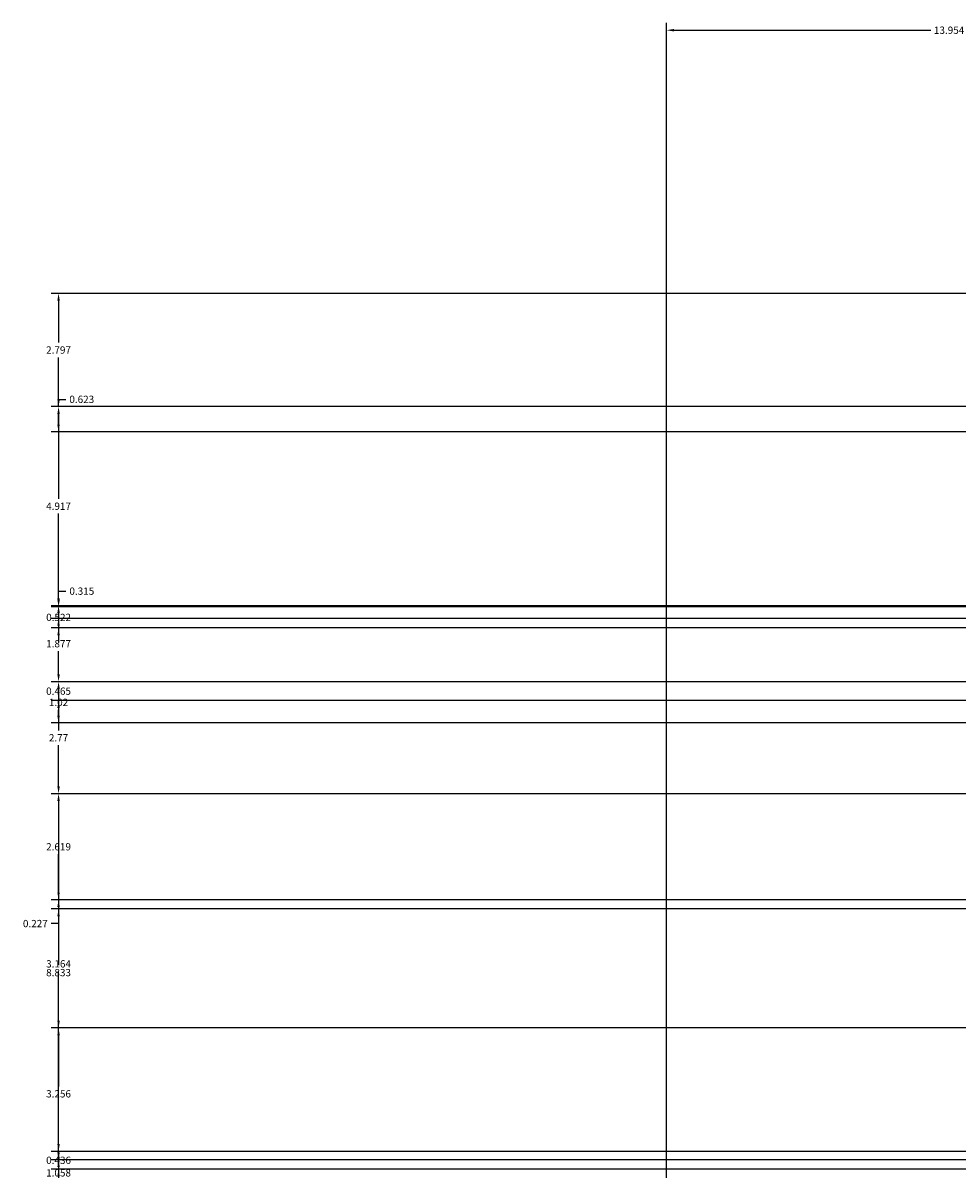
# Model space of a CAD drawing. Units: inches. Extents: x -10 to 130, y -32 to 34.
# Tile 5 of 22: x -10 to 13, y 6 to 34. Entities that reach past the tile are written whole.
import ezdxf

# ---------------------------------------------------------------- set-up
doc = ezdxf.new("R2010")
doc.units = ezdxf.units.IN
doc.header["$MEASUREMENT"] = 0
doc.layers.add('A-ANNO-DIMS', color=2, linetype='Continuous', lineweight=18)
doc.styles.get("Standard").update_dxf_attribs({"font": 'arial.ttf'})
doc.dimstyles.get("Standard").update_dxf_attribs({"dimtxt": 0.18, "dimasz": 0.18, "dimexe": 0.18, "dimexo": 0.0625, "dimgap": 0.09, "dimtad": 0, "dimtih": 1, "dimtoh": 1, "dimdec": 4, "dimzin": 0, "dimdsep": 46, "dimtxsty": 'Standard', "dimcen": 0.09, "dimadec": 0, "dimazin": 0, "dimtfac": 1, "dimtdec": 4, "dimtofl": 0, "dimtmove": 0, "dimatfit": 3, "dimfxl": 1, "dimtolj": 1, "dimtzin": 0, "dimarcsym": 0})

# ---------------------------------------------------------------- blocks, each defined once
blk = doc.blocks.new('*D11')
at = {"layer": 'A-ANNO-DIMS', "color": 0, "lineweight": -2, "transparency": 16777216}
for p, q in [((5.634, -12.739), (5.634, 33.879)), ((5.814, 33.699), (12.156, 33.699)), ((19.408, 33.699), (13.066, 33.699)), ((19.588, 19.547), (19.588, 33.879))]:
    blk.add_line(p, q, dxfattribs=at)
at = {"layer": 'A-ANNO-DIMS', "color": 0, "transparency": 16777216}
for points in [[(5.814, 33.729), (5.814, 33.669), (5.634, 33.699)], [(19.408, 33.729), (19.408, 33.669), (19.588, 33.699)]]:
    blk.add_solid(points, dxfattribs=at)
at = {"layer": 'Defpoints', "color": 0, "transparency": 16777216}
for p in [(19.588, 33.699), (19.588, 19.485), (5.634, -12.801)]:
    blk.add_point(p, dxfattribs=at)
at = {"layer": 'A-ANNO-DIMS', "color": 0, "transparency": 16777216, "insert": (12.611, 33.699), "char_height": 0.18, "attachment_point": 5}
blk.add_mtext('\\A1;13.954', dxfattribs=at)
blk = doc.blocks.new('*D34')
at = {"layer": 'A-ANNO-DIMS', "color": 0, "lineweight": -2, "transparency": 16777216}
for p, q in [((13.34, 6.007), (-9.564, 6.007)), ((-9.384, 5.827), (-9.384, 3.941)), ((-9.384, 1.691), (-9.384, 3.577)), ((70.835, 1.511), (-9.564, 1.511))]:
    blk.add_line(p, q, dxfattribs=at)
at = {"layer": 'A-ANNO-DIMS', "color": 0, "transparency": 16777216}
for points in [[(-9.414, 5.827), (-9.354, 5.827), (-9.384, 6.007)], [(-9.414, 1.691), (-9.354, 1.691), (-9.384, 1.511)]]:
    blk.add_solid(points, dxfattribs=at)
at = {"layer": 'Defpoints', "color": 0, "transparency": 16777216}
for p in [(-9.384, 6.007), (13.402, 6.007), (70.898, 1.511)]:
    blk.add_point(p, dxfattribs=at)
at = {"layer": 'A-ANNO-DIMS', "color": 0, "transparency": 16777216, "insert": (-9.384, 3.759), "char_height": 0.18, "attachment_point": 5}
blk.add_mtext('\\A1;4.497', dxfattribs=at)
blk = doc.blocks.new('*D35')
at = {"layer": 'A-ANNO-DIMS', "color": 0, "lineweight": -2, "transparency": 16777216}
for p, q in [((21.653, 14.841), (-9.564, 14.841)), ((-9.384, 14.661), (-9.384, 10.606)), ((-9.384, 6.187), (-9.384, 10.242)), ((13.34, 6.007), (-9.564, 6.007))]:
    blk.add_line(p, q, dxfattribs=at)
at = {"layer": 'A-ANNO-DIMS', "color": 0, "transparency": 16777216}
for points in [[(-9.414, 14.661), (-9.354, 14.661), (-9.384, 14.841)], [(-9.414, 6.187), (-9.354, 6.187), (-9.384, 6.007)]]:
    blk.add_solid(points, dxfattribs=at)
at = {"layer": 'Defpoints', "color": 0, "transparency": 16777216}
for p in [(-9.384, 14.841), (21.715, 14.841), (13.402, 6.007)]:
    blk.add_point(p, dxfattribs=at)
at = {"layer": 'A-ANNO-DIMS', "color": 0, "transparency": 16777216, "insert": (-9.384, 10.424), "char_height": 0.18, "attachment_point": 5}
blk.add_mtext('\\A1;8.833', dxfattribs=at)
blk = doc.blocks.new('*D36')
at = {"layer": 'A-ANNO-DIMS', "color": 0, "lineweight": -2, "transparency": 16777216}
for p, q in [((44.559, 17.607), (-9.564, 17.607)), ((-9.384, 17.427), (-9.384, 16.405)), ((-9.384, 15.021), (-9.384, 16.044)), ((21.653, 14.841), (-9.564, 14.841))]:
    blk.add_line(p, q, dxfattribs=at)
at = {"layer": 'A-ANNO-DIMS', "color": 0, "transparency": 16777216}
for points in [[(-9.414, 17.427), (-9.354, 17.427), (-9.384, 17.607)], [(-9.414, 15.021), (-9.354, 15.021), (-9.384, 14.841)]]:
    blk.add_solid(points, dxfattribs=at)
at = {"layer": 'Defpoints', "color": 0, "transparency": 16777216}
for p in [(-9.384, 17.607), (44.622, 17.607), (21.715, 14.841)]:
    blk.add_point(p, dxfattribs=at)
at = {"layer": 'A-ANNO-DIMS', "color": 0, "transparency": 16777216, "insert": (-9.384, 16.224), "char_height": 0.18, "attachment_point": 5}
blk.add_mtext('\\A1;2.77', dxfattribs=at)
blk = doc.blocks.new('*D37')
at = {"layer": 'A-ANNO-DIMS', "color": 0, "lineweight": -2, "transparency": 16777216}
for p, q in [((19.526, 19.485), (-9.564, 19.485)), ((-9.384, 19.305), (-9.384, 18.728)), ((-9.384, 17.787), (-9.384, 18.364)), ((44.559, 17.607), (-9.564, 17.607))]:
    blk.add_line(p, q, dxfattribs=at)
at = {"layer": 'A-ANNO-DIMS', "color": 0, "transparency": 16777216}
for points in [[(-9.414, 19.305), (-9.354, 19.305), (-9.384, 19.485)], [(-9.414, 17.787), (-9.354, 17.787), (-9.384, 17.607)]]:
    blk.add_solid(points, dxfattribs=at)
at = {"layer": 'Defpoints', "color": 0, "transparency": 16777216}
for p in [(-9.384, 19.485), (19.588, 19.485), (44.622, 17.607)]:
    blk.add_point(p, dxfattribs=at)
at = {"layer": 'A-ANNO-DIMS', "color": 0, "transparency": 16777216, "insert": (-9.384, 18.546), "char_height": 0.18, "attachment_point": 5}
blk.add_mtext('\\A1;1.877', dxfattribs=at)
blk = doc.blocks.new('*D38')
at = {"layer": 'A-ANNO-DIMS', "color": 0, "lineweight": -2, "transparency": 16777216}
for p, q in [((28.037, 24.402), (-9.564, 24.402)), ((-9.384, 24.222), (-9.384, 22.125)), ((-9.384, 19.665), (-9.384, 21.761)), ((19.526, 19.485), (-9.564, 19.485))]:
    blk.add_line(p, q, dxfattribs=at)
at = {"layer": 'A-ANNO-DIMS', "color": 0, "transparency": 16777216}
for points in [[(-9.414, 24.222), (-9.354, 24.222), (-9.384, 24.402)], [(-9.414, 19.665), (-9.354, 19.665), (-9.384, 19.485)]]:
    blk.add_solid(points, dxfattribs=at)
at = {"layer": 'Defpoints', "color": 0, "transparency": 16777216}
for p in [(-9.384, 24.402), (28.1, 24.402), (19.588, 19.485)]:
    blk.add_point(p, dxfattribs=at)
at = {"layer": 'A-ANNO-DIMS', "color": 0, "transparency": 16777216, "insert": (-9.384, 21.943), "char_height": 0.18, "attachment_point": 5}
blk.add_mtext('\\A1;4.917', dxfattribs=at)
blk = doc.blocks.new('*D39')
at = {"layer": 'A-ANNO-DIMS', "color": 0, "lineweight": -2, "transparency": 16777216}
for p, q in [((49.972, 27.199), (-9.564, 27.199)), ((-9.384, 27.019), (-9.384, 25.982)), ((-9.384, 24.582), (-9.384, 25.618)), ((28.037, 24.402), (-9.564, 24.402))]:
    blk.add_line(p, q, dxfattribs=at)
at = {"layer": 'A-ANNO-DIMS', "color": 0, "transparency": 16777216}
for points in [[(-9.414, 27.019), (-9.354, 27.019), (-9.384, 27.199)], [(-9.414, 24.582), (-9.354, 24.582), (-9.384, 24.402)]]:
    blk.add_solid(points, dxfattribs=at)
at = {"layer": 'Defpoints', "color": 0, "transparency": 16777216}
for p in [(-9.384, 27.199), (50.035, 27.199), (28.1, 24.402)]:
    blk.add_point(p, dxfattribs=at)
at = {"layer": 'A-ANNO-DIMS', "color": 0, "transparency": 16777216, "insert": (-9.384, 25.8), "char_height": 0.18, "attachment_point": 5}
blk.add_mtext('\\A1;2.797', dxfattribs=at)
blk = doc.blocks.new('*D74')
at = {"layer": 'A-ANNO-DIMS', "color": 0, "lineweight": -2, "transparency": 16777216}
for p, q in [((54.085, 17.607), (-9.564, 17.607)), ((-9.384, 17.427), (-9.384, 17.281)), ((-9.384, 16.771), (-9.384, 16.917)), ((55.856, 16.591), (-9.564, 16.591))]:
    blk.add_line(p, q, dxfattribs=at)
at = {"layer": 'A-ANNO-DIMS', "color": 0, "transparency": 16777216}
for points in [[(-9.414, 17.427), (-9.354, 17.427), (-9.384, 17.607)], [(-9.414, 16.771), (-9.354, 16.771), (-9.384, 16.591)]]:
    blk.add_solid(points, dxfattribs=at)
at = {"layer": 'Defpoints', "color": 0, "transparency": 16777216}
for p in [(54.147, 17.607), (-9.384, 16.591), (55.918, 16.591)]:
    blk.add_point(p, dxfattribs=at)
at = {"layer": 'A-ANNO-DIMS', "color": 0, "transparency": 16777216, "insert": (-9.384, 17.099), "char_height": 0.18, "attachment_point": 5}
blk.add_mtext('\\A1;1.02', dxfattribs=at)
blk = doc.blocks.new('*D87')
at = {"layer": 'A-ANNO-DIMS', "color": 0, "lineweight": -2, "transparency": 16777216}
for p, q in [((49.884, 14.841), (-9.564, 14.841)), ((-9.384, 14.661), (-9.384, 13.713)), ((-9.384, 12.402), (-9.384, 13.35)), ((49.884, 12.222), (-9.564, 12.222))]:
    blk.add_line(p, q, dxfattribs=at)
at = {"layer": 'A-ANNO-DIMS', "color": 0, "transparency": 16777216}
for points in [[(-9.414, 14.661), (-9.354, 14.661), (-9.384, 14.841)], [(-9.414, 12.402), (-9.354, 12.402), (-9.384, 12.222)]]:
    blk.add_solid(points, dxfattribs=at)
at = {"layer": 'Defpoints', "color": 0, "transparency": 16777216}
for p in [(49.946, 14.841), (-9.384, 12.222), (49.946, 12.222)]:
    blk.add_point(p, dxfattribs=at)
at = {"layer": 'A-ANNO-DIMS', "color": 0, "transparency": 16777216, "insert": (-9.384, 13.532), "char_height": 0.18, "attachment_point": 5}
blk.add_mtext('\\A1;2.619', dxfattribs=at)
blk = doc.blocks.new('*D88')
at = {"layer": 'A-ANNO-DIMS', "color": 0, "lineweight": -2, "transparency": 16777216}
for p, q in [((49.884, 12.222), (-9.564, 12.222)), ((-9.384, 12.042), (-9.384, 10.822)), ((-9.384, 9.238), (-9.384, 10.458)), ((49.884, 9.058), (-9.564, 9.058))]:
    blk.add_line(p, q, dxfattribs=at)
at = {"layer": 'A-ANNO-DIMS', "color": 0, "transparency": 16777216}
for points in [[(-9.414, 12.042), (-9.354, 12.042), (-9.384, 12.222)], [(-9.414, 9.238), (-9.354, 9.238), (-9.384, 9.058)]]:
    blk.add_solid(points, dxfattribs=at)
at = {"layer": 'Defpoints', "color": 0, "transparency": 16777216}
for p in [(49.946, 12.222), (-9.384, 9.058), (49.946, 9.058)]:
    blk.add_point(p, dxfattribs=at)
at = {"layer": 'A-ANNO-DIMS', "color": 0, "transparency": 16777216, "insert": (-9.384, 10.64), "char_height": 0.18, "attachment_point": 5}
blk.add_mtext('\\A1;3.164', dxfattribs=at)
blk = doc.blocks.new('*D89')
at = {"layer": 'A-ANNO-DIMS', "color": 0, "lineweight": -2, "transparency": 16777216}
for p, q in [((49.884, 9.058), (-9.564, 9.058)), ((-9.384, 8.878), (-9.384, 7.612)), ((-9.384, 5.982), (-9.384, 7.248)), ((49.884, 5.802), (-9.564, 5.802))]:
    blk.add_line(p, q, dxfattribs=at)
at = {"layer": 'A-ANNO-DIMS', "color": 0, "transparency": 16777216}
for points in [[(-9.414, 8.878), (-9.354, 8.878), (-9.384, 9.058)], [(-9.414, 5.982), (-9.354, 5.982), (-9.384, 5.802)]]:
    blk.add_solid(points, dxfattribs=at)
at = {"layer": 'Defpoints', "color": 0, "transparency": 16777216}
for p in [(49.946, 9.058), (-9.384, 5.802), (49.946, 5.802)]:
    blk.add_point(p, dxfattribs=at)
at = {"layer": 'A-ANNO-DIMS', "color": 0, "transparency": 16777216, "insert": (-9.384, 7.43), "char_height": 0.18, "attachment_point": 5}
blk.add_mtext('\\A1;3.256', dxfattribs=at)
blk = doc.blocks.new('*D90')
at = {"layer": 'A-ANNO-DIMS', "color": 0, "lineweight": -2, "transparency": 16777216}
for p, q in [((49.884, 5.802), (-9.564, 5.802)), ((-9.384, 5.622), (-9.384, 4.421)), ((-9.384, 2.855), (-9.384, 4.057)), ((49.884, 2.675), (-9.564, 2.675))]:
    blk.add_line(p, q, dxfattribs=at)
at = {"layer": 'A-ANNO-DIMS', "color": 0, "transparency": 16777216}
for points in [[(-9.414, 5.622), (-9.354, 5.622), (-9.384, 5.802)], [(-9.414, 2.855), (-9.354, 2.855), (-9.384, 2.675)]]:
    blk.add_solid(points, dxfattribs=at)
at = {"layer": 'Defpoints', "color": 0, "transparency": 16777216}
for p in [(49.946, 5.802), (-9.384, 2.675), (49.946, 2.675)]:
    blk.add_point(p, dxfattribs=at)
at = {"layer": 'A-ANNO-DIMS', "color": 0, "transparency": 16777216, "insert": (-9.384, 4.239), "char_height": 0.18, "attachment_point": 5}
blk.add_mtext('\\A1;3.127', dxfattribs=at)
blk = doc.blocks.new('*D95')
at = {"layer": 'A-ANNO-DIMS', "color": 0, "lineweight": -2, "transparency": 16777216}
for p, q in [((-9.384, 12.402), (-9.384, 12.582)), ((49.884, 12.222), (-9.564, 12.222)), ((49.884, 11.995), (-9.564, 11.995)), ((-9.384, 11.635), (-9.564, 11.635)), ((-9.384, 11.815), (-9.384, 11.635))]:
    blk.add_line(p, q, dxfattribs=at)
at = {"layer": 'A-ANNO-DIMS', "color": 0, "transparency": 16777216}
for points in [[(-9.414, 12.402), (-9.354, 12.402), (-9.384, 12.222)], [(-9.414, 11.815), (-9.354, 11.815), (-9.384, 11.995)]]:
    blk.add_solid(points, dxfattribs=at)
at = {"layer": 'Defpoints', "color": 0, "transparency": 16777216}
for p in [(49.946, 12.222), (-9.384, 11.995), (49.946, 11.995)]:
    blk.add_point(p, dxfattribs=at)
at = {"layer": 'A-ANNO-DIMS', "color": 0, "transparency": 16777216, "insert": (-9.957, 11.635), "char_height": 0.18, "attachment_point": 5}
blk.add_mtext('\\A1;0.227', dxfattribs=at)
blk = doc.blocks.new('*D98')
at = {"layer": 'A-ANNO-DIMS', "color": 0, "lineweight": -2, "transparency": 16777216}
for p, q in [((-9.384, 19.665), (-9.384, 19.845)), ((-9.384, 19.845), (-9.204, 19.845)), ((19.526, 19.485), (-9.564, 19.485)), ((19.785, 19.17), (-9.564, 19.17)), ((-9.384, 18.99), (-9.384, 18.81))]:
    blk.add_line(p, q, dxfattribs=at)
at = {"layer": 'A-ANNO-DIMS', "color": 0, "transparency": 16777216}
for points in [[(-9.414, 19.665), (-9.354, 19.665), (-9.384, 19.485)], [(-9.414, 18.99), (-9.354, 18.99), (-9.384, 19.17)]]:
    blk.add_solid(points, dxfattribs=at)
at = {"layer": 'Defpoints', "color": 0, "transparency": 16777216}
for p in [(-9.384, 19.485), (19.588, 19.485), (19.848, 19.17)]:
    blk.add_point(p, dxfattribs=at)
at = {"layer": 'A-ANNO-DIMS', "color": 0, "transparency": 16777216, "insert": (-8.809, 19.845), "char_height": 0.18, "attachment_point": 5}
blk.add_mtext('\\A1;0.315', dxfattribs=at)
blk = doc.blocks.new('*D101')
at = {"layer": 'A-ANNO-DIMS', "color": 0, "lineweight": -2, "transparency": 16777216}
for p, q in [((28.037, 24.402), (-9.564, 24.402)), ((-9.384, 24.402), (-9.384, 24.582)), ((-9.384, 24.582), (-9.204, 24.582)), ((-9.384, 23.959), (-9.384, 24.222)), ((28.602, 23.779), (-9.564, 23.779))]:
    blk.add_line(p, q, dxfattribs=at)
at = {"layer": 'A-ANNO-DIMS', "color": 0, "transparency": 16777216}
for points in [[(-9.414, 24.222), (-9.354, 24.222), (-9.384, 24.402)], [(-9.414, 23.959), (-9.354, 23.959), (-9.384, 23.779)]]:
    blk.add_solid(points, dxfattribs=at)
at = {"layer": 'Defpoints', "color": 0, "transparency": 16777216}
for p in [(-9.384, 24.402), (28.1, 24.402), (28.665, 23.779)]:
    blk.add_point(p, dxfattribs=at)
at = {"layer": 'A-ANNO-DIMS', "color": 0, "transparency": 16777216, "insert": (-8.81, 24.582), "char_height": 0.18, "attachment_point": 5}
blk.add_mtext('\\A1;0.623', dxfattribs=at)
blk = doc.blocks.new('*D104')
at = {"layer": 'A-ANNO-DIMS', "color": 0, "lineweight": -2, "transparency": 16777216}
for p, q in [((-9.383551, 19.637521), (-9.383551, 19.817521)), ((33.54566, 19.457521), (-9.563551, 19.457521)), ((33.931459, 18.935883), (-9.563551, 18.935883)), ((-9.383551, 18.755883), (-9.383551, 18.575883))]:
    blk.add_line(p, q, dxfattribs=at)
at = {"layer": 'A-ANNO-DIMS', "color": 0, "transparency": 16777216}
for points in [[(-9.413551, 19.637521), (-9.353551, 19.637521), (-9.383551, 19.457521)], [(-9.413551, 18.755883), (-9.353551, 18.755883), (-9.383551, 18.935883)]]:
    blk.add_solid(points, dxfattribs=at)
at = {"layer": 'Defpoints', "color": 0, "transparency": 16777216}
for p in [(-9.383551, 19.457521), (33.60816, 19.457521), (33.993959, 18.935883)]:
    blk.add_point(p, dxfattribs=at)
at = {"layer": 'A-ANNO-DIMS', "color": 0, "transparency": 16777216, "insert": (-9.383551, 19.196702), "char_height": 0.18, "attachment_point": 5}
blk.add_mtext('\\A1;0.522', dxfattribs=at)
blk = doc.blocks.new('*D110')
at = {"layer": 'A-ANNO-DIMS', "color": 0, "lineweight": -2, "transparency": 16777216}
for p, q in [((-9.383551, 17.787359), (-9.383551, 17.967359)), ((44.559228, 17.607359), (-9.563551, 17.607359)), ((45.040057, 17.142679), (-9.563551, 17.142679)), ((-9.383551, 16.962679), (-9.383551, 16.782679))]:
    blk.add_line(p, q, dxfattribs=at)
at = {"layer": 'A-ANNO-DIMS', "color": 0, "transparency": 16777216}
for points in [[(-9.413551, 17.787359), (-9.353551, 17.787359), (-9.383551, 17.607359)], [(-9.413551, 16.962679), (-9.353551, 16.962679), (-9.383551, 17.142679)]]:
    blk.add_solid(points, dxfattribs=at)
at = {"layer": 'Defpoints', "color": 0, "transparency": 16777216}
for p in [(-9.383551, 17.607359), (44.621728, 17.607359), (45.102557, 17.142679)]:
    blk.add_point(p, dxfattribs=at)
at = {"layer": 'A-ANNO-DIMS', "color": 0, "transparency": 16777216, "insert": (-9.383551, 17.375019), "char_height": 0.18, "attachment_point": 5}
blk.add_mtext('\\A1;0.465', dxfattribs=at)
blk = doc.blocks.new('*D113')
at = {"layer": 'A-ANNO-DIMS', "color": 0, "lineweight": -2, "transparency": 16777216}
for p, q in [((13.34, 6.007), (-9.564, 6.007)), ((-9.384, 5.827), (-9.384, 5.66)), ((-9.384, 5.13), (-9.384, 5.297)), ((14.67, 4.95), (-9.564, 4.95))]:
    blk.add_line(p, q, dxfattribs=at)
at = {"layer": 'A-ANNO-DIMS', "color": 0, "transparency": 16777216}
for points in [[(-9.414, 5.827), (-9.354, 5.827), (-9.384, 6.007)], [(-9.414, 5.13), (-9.354, 5.13), (-9.384, 4.95)]]:
    blk.add_solid(points, dxfattribs=at)
at = {"layer": 'Defpoints', "color": 0, "transparency": 16777216}
for p in [(-9.384, 6.007), (13.402, 6.007), (14.732, 4.95)]:
    blk.add_point(p, dxfattribs=at)
at = {"layer": 'A-ANNO-DIMS', "color": 0, "transparency": 16777216, "insert": (-9.384, 5.478), "char_height": 0.18, "attachment_point": 5}
blk.add_mtext('\\A1;1.058', dxfattribs=at)
blk = doc.blocks.new('*D115')
at = {"layer": 'A-ANNO-DIMS', "color": 0, "lineweight": -2, "transparency": 16777216}
for p, q in [((26.336, 6.007), (-9.564, 6.007)), ((-9.384, 5.827), (-9.384, 4.151)), ((-9.384, 2.111), (-9.384, 3.787)), ((26.336, 1.931), (-9.564, 1.931))]:
    blk.add_line(p, q, dxfattribs=at)
at = {"layer": 'A-ANNO-DIMS', "color": 0, "transparency": 16777216}
for points in [[(-9.414, 5.827), (-9.354, 5.827), (-9.384, 6.007)], [(-9.414, 2.111), (-9.354, 2.111), (-9.384, 1.931)]]:
    blk.add_solid(points, dxfattribs=at)
at = {"layer": 'Defpoints', "color": 0, "transparency": 16777216}
for p in [(26.399, 6.007), (-9.384, 1.931), (26.399, 1.931)]:
    blk.add_point(p, dxfattribs=at)
at = {"layer": 'A-ANNO-DIMS', "color": 0, "transparency": 16777216, "insert": (-9.384, 3.969), "char_height": 0.18, "attachment_point": 5}
blk.add_mtext('\\A1;4.076', dxfattribs=at)
blk = doc.blocks.new('*D121')
at = {"layer": 'A-ANNO-DIMS', "color": 0, "lineweight": -2, "transparency": 16777216}
for p, q in [((-9.384, 6.187), (-9.384, 6.367)), ((31.909, 6.007), (-9.564, 6.007)), ((32.427, 5.572), (-9.564, 5.572)), ((-9.384, 5.392), (-9.384, 5.212))]:
    blk.add_line(p, q, dxfattribs=at)
at = {"layer": 'A-ANNO-DIMS', "color": 0, "transparency": 16777216}
for points in [[(-9.414, 6.187), (-9.354, 6.187), (-9.384, 6.007)], [(-9.414, 5.392), (-9.354, 5.392), (-9.384, 5.572)]]:
    blk.add_solid(points, dxfattribs=at)
at = {"layer": 'Defpoints', "color": 0, "transparency": 16777216}
for p in [(-9.384, 6.007), (31.971, 6.007), (32.49, 5.572)]:
    blk.add_point(p, dxfattribs=at)
at = {"layer": 'A-ANNO-DIMS', "color": 0, "transparency": 16777216, "insert": (-9.384, 5.789), "char_height": 0.18, "attachment_point": 5}
blk.add_mtext('\\A1;0.436', dxfattribs=at)

msp = doc.modelspace()

# ---------------------------------------------------------------- dimensions: what is measured, and where the dimension line sits
at = {"layer": 'A-ANNO-DIMS'}
dim = msp.add_linear_dim(base=(19.5881, 33.6987), p1=(5.634, -12.8012), p2=(19.5881, 19.4845), dimstyle='Standard', override={"dimdec": 3, "dimlfac": 1, "dimrnd": 0, "dimzin": 0, "dimdsep": 46, "dimlunit": 2}, dxfattribs=at)
dim.commit()
dim.dimension.update_dxf_attribs({"geometry": '*D11', "text_midpoint": (12.611, 33.6987)})
for base, p1, p2, override, picture, middle in [((-9.3836, 27.1987), (28.0997, 24.4019), (50.0347, 27.1987), {"dimdec": 3, "dimlfac": 1, "dimrnd": 0, "dimzin": 0, "dimdsep": 46, "dimlunit": 2}, '*D39', (-9.3836, 25.8003)), ((-9.3836, 24.4019), (28.6645, 23.7785), (28.0997, 24.4019), {"dimdec": 3, "dimlfac": 1, "dimrnd": 0, "dimzin": 0, "dimdsep": 46, "dimlunit": 2}, '*D101', (-8.8098, 24.5819)), ((-9.3836, 24.4019), (19.5881, 19.4845), (28.0997, 24.4019), {"dimdec": 3, "dimlfac": 1, "dimrnd": 0, "dimzin": 0, "dimdsep": 46, "dimlunit": 2}, '*D38', (-9.3836, 21.9432)), ((-9.3836, 19.4575), (33.994, 18.9359), (33.6082, 19.4575), {"dimdec": 3, "dimlfac": 1, "dimrnd": 0, "dimzin": 0, "dimdsep": 46, "dimlunit": 2}, '*D104', (-9.3836, 19.1967)), ((-9.3836, 19.4845), (19.8477, 19.1697), (19.5881, 19.4845), {"dimdec": 3, "dimlfac": 1, "dimrnd": 0, "dimzin": 0, "dimdsep": 46, "dimlunit": 2}, '*D98', (-8.8092, 19.8445)), ((-9.3836, 19.4845), (44.6217, 17.6074), (19.5881, 19.4845), {"dimdec": 3, "dimlfac": 1, "dimrnd": 0, "dimzin": 0, "dimdsep": 46, "dimlunit": 2}, '*D37', (-9.3836, 18.5459)), ((-9.3836, 17.6074), (45.1026, 17.1427), (44.6217, 17.6074), {"dimdec": 3, "dimlfac": 1, "dimrnd": 0, "dimzin": 0, "dimdsep": 46, "dimlunit": 2}, '*D110', (-9.3836, 17.375)), ((-9.3836, 17.6074), (21.7155, 14.8409), (44.6217, 17.6074), {"dimdec": 2, "dimlfac": 1, "dimrnd": 0, "dimzin": 0, "dimdsep": 46, "dimlunit": 2}, '*D36', (-9.3836, 16.2241)), ((-9.3836, 16.5911), (54.1471, 17.6074), (55.9182, 16.5911), {"dimdec": 2, "dimlfac": 1, "dimrnd": 0, "dimzin": 0, "dimdsep": 46, "dimlunit": 2}, '*D74', (-9.3836, 17.0992)), ((-9.383551, 14.84094), (13.402105, 6.007442), (21.715452, 14.84094), {"dimdec": 3, "dimlfac": 1, "dimrnd": 0, "dimzin": 0, "dimdsep": 46, "dimlunit": 2}, '*D35', (-9.383551, 10.424191)), ((-9.3836, 12.2222), (49.9462, 14.8409), (49.9462, 12.2222), {"dimdec": 3, "dimlfac": 1, "dimrnd": 0, "dimzin": 0, "dimdsep": 46, "dimlunit": 2}, '*D87', (-9.3836, 13.5316)), ((-9.3836, 11.9951), (49.9462, 12.2222), (49.9462, 11.9951), {"dimdec": 3, "dimlfac": 1, "dimrnd": 0, "dimzin": 0, "dimdsep": 46, "dimlunit": 2}, '*D95', (-9.9573, 11.6351)), ((-9.3836, 9.058), (49.9462, 12.2222), (49.9462, 9.058), {"dimdec": 3, "dimlfac": 1, "dimrnd": 0, "dimzin": 0, "dimdsep": 46, "dimlunit": 2}, '*D88', (-9.3836, 10.6401)), ((-9.3836, 5.8024), (49.9462, 9.058), (49.9462, 5.8024), {"dimdec": 3, "dimlfac": 1, "dimrnd": 0, "dimzin": 0, "dimdsep": 46, "dimlunit": 2}, '*D89', (-9.3836, 7.4302)), ((-9.3836, 6.0074), (32.4898, 5.5715), (31.9712, 6.0074), {"dimdec": 3, "dimlfac": 1, "dimrnd": 0, "dimzin": 0, "dimdsep": 46, "dimlunit": 2}, '*D121', (-9.3836, 5.7895)), ((-9.3836, 6.0074), (70.898, 1.5107), (13.4021, 6.0074), {"dimdec": 3, "dimlfac": 1, "dimrnd": 0, "dimzin": 0, "dimdsep": 46, "dimlunit": 2}, '*D34', (-9.3836, 3.7591)), ((-9.3836, 6.0074), (14.7324, 4.9495), (13.4021, 6.0074), {"dimdec": 3, "dimlfac": 1, "dimrnd": 0, "dimzin": 0, "dimdsep": 46, "dimlunit": 2}, '*D113', (-9.3836, 5.4785)), ((-9.3836, 1.931), (26.3988, 6.0074), (26.3988, 1.931), {"dimdec": 3, "dimlfac": 1, "dimrnd": 0, "dimzin": 0, "dimdsep": 46, "dimlunit": 2}, '*D115', (-9.3836, 3.9692)), ((-9.3836, 2.6753), (49.9462, 5.8024), (49.9462, 2.6753), {"dimdec": 3, "dimlfac": 1, "dimrnd": 0, "dimzin": 0, "dimdsep": 46, "dimlunit": 2}, '*D90', (-9.3836, 4.2388))]:
    dim = msp.add_linear_dim(base=base, p1=p1, p2=p2, angle=90, dimstyle='Standard', override=override, dxfattribs=at)
    dim.commit()
    dim.dimension.update_dxf_attribs({"geometry": picture, "text_midpoint": middle})

doc.saveas('drawing.dxf')
